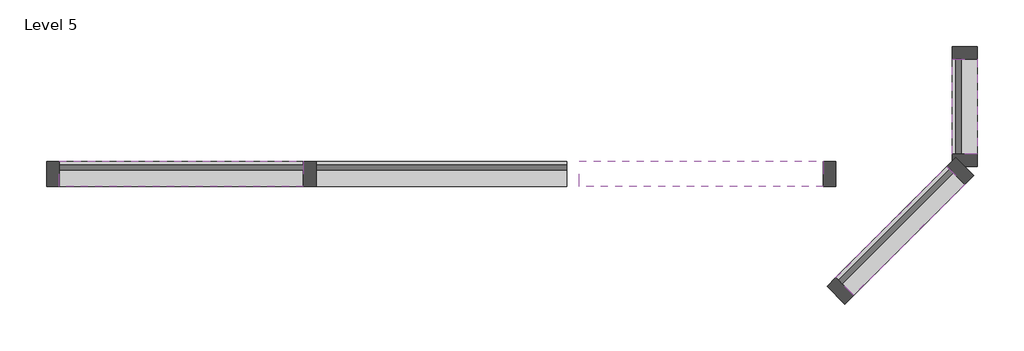
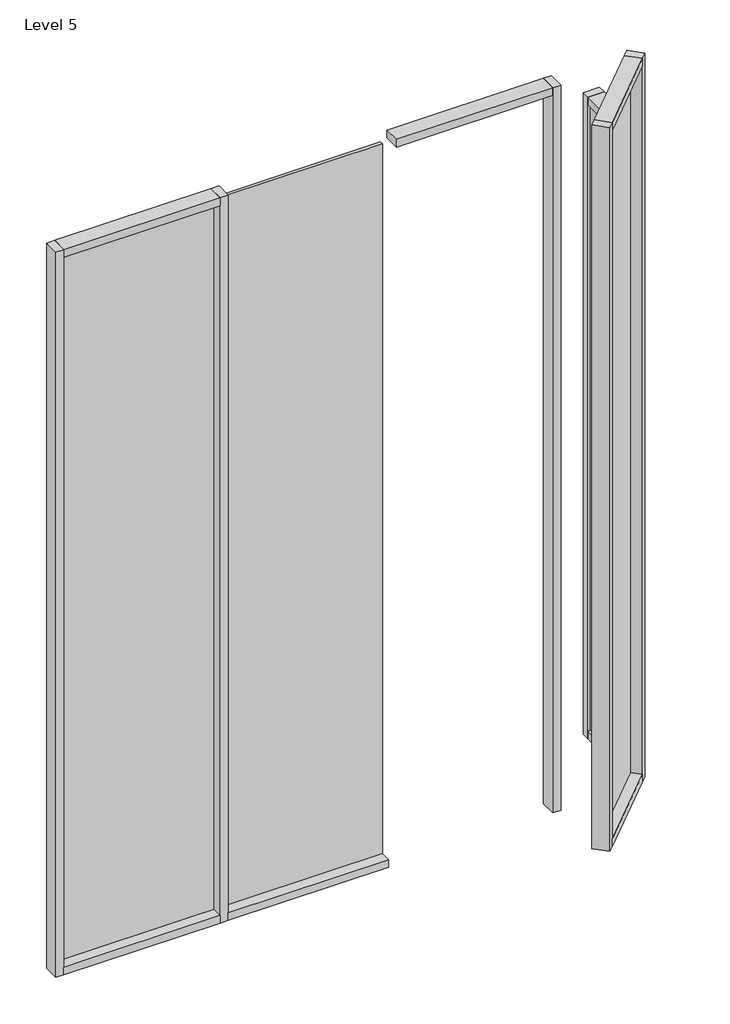
# One storey: 15 members, 4 plates.
"""IFC4 building model written with IfcOpenShell, lengths in millimetres."""

from ifc_helpers import new_model, si_unit, origin, place, context, project, spatial, transform, mapped, element, save
from components import member_3728dc7a, member_6c8266e2, member_429f6687, member_74cc3c14, member_ecd02cc6, member_aa97c3f9, member_9771a04b, member_bcb6a316, system_panel_glazed_aa365302, system_panel_glazed_f7b0ce0e, system_panel_glazed_d8816065, system_panel_glazed_3f11bb86

model = new_model("IFC4")

# Units and contexts
model_context = context("Model", 3, world=origin())
ifc_project = project(units=[si_unit("LENGTHUNIT", "METRE", prefix="MILLI")], contexts=[model_context])

# Site, building, storey
site = spatial("IfcSite", under=ifc_project)
building = spatial("IfcBuilding", under=site)
storey = spatial("IfcBuildingStorey", under=building, Name="Level 5", Elevation=12192.0)

# Members
placement = place(None, origin())
member_shape = member_3728dc7a(model_context)
element("IfcMember", 1, ObjectType="Rectangular Mullion : 2.5\" x 5\" rectangular", at=placement, inside=storey, context=model_context, shape_type="MappedRepresentation", body=[
    mapped(member_shape, transform((-8905.5233471, 9418.207593, 15680.745847), x_axis=(0.0, 0.0, 1.0), y_axis=(1.0, 0.0, 0.0), z_axis=(0.0, 1.0, 0.0))),
])
element("IfcMember", 2, ObjectType="Rectangular Mullion : 2.5\" x 5\" rectangular", at=placement, inside=storey, context=model_context, shape_type="MappedRepresentation", body=[
    mapped(member_shape, transform((-8905.5233471, 8941.5592809, 10363.2), x_axis=(0.0, 0.0, -1.0), y_axis=(1.0, 0.0, 0.0), z_axis=(0.0, -1.0, 0.0))),
])
member_2_shape = member_6c8266e2(model_context)
element("IfcMember", 3, ObjectType="Rectangular Mullion : 2.5\" x 5\" rectangular", at=placement, inside=storey, context=model_context, shape_type="MappedRepresentation", body=[
    mapped(member_2_shape, transform((-8905.5233471, 9481.707593, 10363.2), x_axis=(0.0, 1.0, 0.0), y_axis=(1.0, 0.0, 0.0), z_axis=(0.0, 0.0, -1.0))),
])
element("IfcMember", 4, ObjectType="Rectangular Mullion : 2.5\" x 5\" rectangular", at=placement, inside=storey, context=model_context, shape_type="MappedRepresentation", body=[
    mapped(member_2_shape, transform((-8905.5233471, 8878.0592809, 15680.745847), x_axis=(0.0, -1.0, 0.0), y_axis=(1.0, 0.0, 0.0), z_axis=(0.0, 0.0, 1.0))),
])
member_3_shape = member_429f6687(model_context)
element("IfcMember", 5, ObjectType="Rectangular Mullion : 2.5\" x 5\" rectangular", at=placement, inside=storey, context=model_context, shape_type="MappedRepresentation", body=[
    mapped(member_3_shape, transform((-8950.4246277, 8833.1580003, 16363.9551516), x_axis=(0.0, 0.0, 1.0), y_axis=(0.7071067811865435, -0.7071067811865517, 0.0), z_axis=(0.7071067811865517, 0.7071067811865435, 0.0))),
])
element("IfcMember", 6, ObjectType="Rectangular Mullion : 2.5\" x 5\" rectangular", at=placement, inside=storey, context=model_context, shape_type="MappedRepresentation", body=[
    mapped(member_3_shape, transform((-9507.2005072, 8276.3821208, 10363.2), x_axis=(0.0, 0.0, -1.0), y_axis=(0.7071067811865435, -0.7071067811865517, 0.0), z_axis=(-0.7071067811865517, -0.7071067811865435, 0.0))),
])
member_4_shape = member_74cc3c14(model_context)
element("IfcMember", 7, ObjectType="Rectangular Mullion : 2.5\" x 5\" rectangular", at=placement, inside=storey, context=model_context, shape_type="MappedRepresentation", body=[
    mapped(member_4_shape, transform((-8905.5233471, 8878.0592809, 10363.2), x_axis=(0.7071067811865518, 0.7071067811865434, 0.0), y_axis=(0.7071067811865434, -0.7071067811865518, 0.0), z_axis=(0.0, 0.0, -1.0))),
])
element("IfcMember", 8, ObjectType="Rectangular Mullion : 2.5\" x 5\" rectangular", at=placement, inside=storey, context=model_context, shape_type="MappedRepresentation", body=[
    mapped(member_4_shape, transform((-9552.1017879, 8231.4808402, 16363.9551516), x_axis=(-0.7071067811865518, -0.7071067811865434, 0.0), y_axis=(0.7071067811865434, -0.7071067811865518, 0.0), z_axis=(0.0, 0.0, 1.0))),
])
member_5_shape = member_ecd02cc6(model_context)
element("IfcMember", 9, ObjectType="Rectangular Mullion : 2.5\" x 5\" rectangular", at=placement, inside=storey, context=model_context, shape_type="MappedRepresentation", body=[
    mapped(member_5_shape, transform((-12193.7017879, 8841.0808402, 10363.2), x_axis=(1.0, 0.0, 0.0), y_axis=(0.0, -1.0, 0.0), z_axis=(0.0, 0.0, -1.0))),
])
member_6_shape = member_aa97c3f9(model_context)
element("IfcMember", 10, ObjectType="Rectangular Mullion : 2.5\" x 5\" rectangular", at=placement, inside=storey, context=model_context, shape_type="MappedRepresentation", body=[
    mapped(member_6_shape, transform((-9552.1017879, 8841.0808402, 10363.2), x_axis=(1.0, 0.0, 0.0), y_axis=(0.0, -1.0, 0.0), z_axis=(0.0, 0.0, -1.0))),
])
element("IfcMember", 11, ObjectType="Rectangular Mullion : 2.5\" x 5\" rectangular", at=placement, inside=storey, context=model_context, shape_type="MappedRepresentation", body=[
    mapped(member_6_shape, transform((-13514.5017879, 8841.0808402, 16374.9116741), x_axis=(-1.0, 0.0, 0.0), y_axis=(0.0, -1.0, 0.0), z_axis=(0.0, 0.0, 1.0))),
])
member_7_shape = member_9771a04b(model_context)
element("IfcMember", 12, ObjectType="Rectangular Mullion : 2.5\" x 5\" rectangular", at=placement, inside=storey, context=model_context, shape_type="MappedRepresentation", body=[
    mapped(member_7_shape, transform((-9615.6017879, 8841.0808402, 16374.9116741), x_axis=(0.0, 0.0, 1.0), y_axis=(0.0, -1.0, 0.0), z_axis=(1.0, 0.0, 0.0))),
])
element("IfcMember", 13, ObjectType="Rectangular Mullion : 2.5\" x 5\" rectangular", at=placement, inside=storey, context=model_context, shape_type="MappedRepresentation", body=[
    mapped(member_7_shape, transform((-12225.4517879, 8841.0808402, 16374.9116741), x_axis=(0.0, 0.0, 1.0), y_axis=(0.0, -1.0, 0.0), z_axis=(1.0, 0.0, 0.0))),
])
element("IfcMember", 14, ObjectType="Rectangular Mullion : 2.5\" x 5\" rectangular", at=placement, inside=storey, context=model_context, shape_type="MappedRepresentation", body=[
    mapped(member_7_shape, transform((-13451.0017879, 8841.0808402, 10363.2), x_axis=(0.0, 0.0, -1.0), y_axis=(0.0, -1.0, 0.0), z_axis=(-1.0, 0.0, 0.0))),
])
member_8_shape = member_bcb6a316(model_context)
element("IfcMember", 15, ObjectType="Rectangular Mullion : 2.5\" x 5\" rectangular", at=placement, inside=storey, context=model_context, shape_type="MappedRepresentation", body=[
    mapped(member_8_shape, transform((-12161.9517879, 8841.0808402, 10363.2), x_axis=(0.0, 0.0, -1.0), y_axis=(0.0, -1.0, 0.0), z_axis=(-1.0, 0.0, 0.0))),
])

# Plates
system_panel_glazed_shape = system_panel_glazed_aa365302(model_context)
element("IfcPlate", 16, ObjectType="System Panel : Glazed", at=placement, inside=storey, context=model_context, shape_type="MappedRepresentation", body=[
    mapped(system_panel_glazed_shape, transform((-8905.5233471, 9179.8834369, 10426.7), x_axis=(0.0, 1.0, 0.0), y_axis=(-1.0, 0.0, 0.0), z_axis=(0.0, 0.0, 1.0))),
])
system_panel_glazed_2_shape = system_panel_glazed_f7b0ce0e(model_context)
element("IfcPlate", 17, ObjectType="System Panel : Glazed", at=placement, inside=storey, context=model_context, shape_type="MappedRepresentation", body=[
    mapped(system_panel_glazed_2_shape, transform((-9228.8125675, 8554.7700605, 10426.7), x_axis=(0.7071067811865518, 0.7071067811865434, 0.0), y_axis=(-0.7071067811865434, 0.7071067811865518, 0.0), z_axis=(0.0, 0.0, 1.0))),
])
system_panel_glazed_3_shape = system_panel_glazed_d8816065(model_context)
element("IfcPlate", 18, ObjectType="System Panel : Glazed", at=placement, inside=storey, context=model_context, shape_type="MappedRepresentation", body=[
    mapped(system_panel_glazed_3_shape, transform((-12838.2267879, 8841.0808402, 10426.7), x_axis=(1.0, 0.0, 0.0), y_axis=(0.0, 1.0, 0.0), z_axis=(0.0, 0.0, 1.0))),
])
system_panel_glazed_4_shape = system_panel_glazed_3f11bb86(model_context)
element("IfcPlate", 19, ObjectType="System Panel : Glazed", at=placement, inside=storey, context=model_context, shape_type="MappedRepresentation", body=[
    mapped(system_panel_glazed_4_shape, transform((-11533.3017879, 8841.0808402, 10426.7), x_axis=(1.0, 0.0, 0.0), y_axis=(0.0, 1.0, 0.0), z_axis=(0.0, 0.0, 1.0))),
])

save(model, "model.ifc")

# Revit data of these elements
# Type "Rectangular Mullion : 2.5\" x 5\" rectangular"
#   built-in parameter 1007304 = 0.416667 (stored number, unit not read)
#   built-in parameter 1007301 = 0.104167 (stored number, unit not read)
#   built-in parameter 1007300 = 0.104167 (stored number, unit not read)
# Type "System Panel : Glazed"
#   Construction Type Id = "GSP4R"
#   Analytic Construction = "1/8 in Pilkington single glazing"
#   Visual Light Transmittance = 0.9
#   Solar Heat Gain Coefficient = 0.86
#   Heat Transfer Coefficient (U) = 1.18115 BTU/(h·ft²·°F)
# Elements 1, 2, 3, 4, 5, 6, 7, 8, 9, 10, 11, 12, 13, 14, 15 (IfcMember, "Rectangular Mullion : 2.5\" x 5\" rectangular")
#   Phase Created = New Construction
#   Materials on its faces: "Iron, Ductile"
# Elements 16, 17, 18, 19 (IfcPlate, "System Panel : Glazed")
#   Phase Created = New Construction
#   Materials on its faces: "Glass"
# Materials
#   "Iron, Ductile": class "Metal", colour RGB 0 0 0, transparency 0, Description = "Ductile cast iron", Cost = 0
#   "Glass": class "Glass", colour RGB 0 128 192, transparency 0.75, Description = "Soda Lime Glass", Cost = 0
